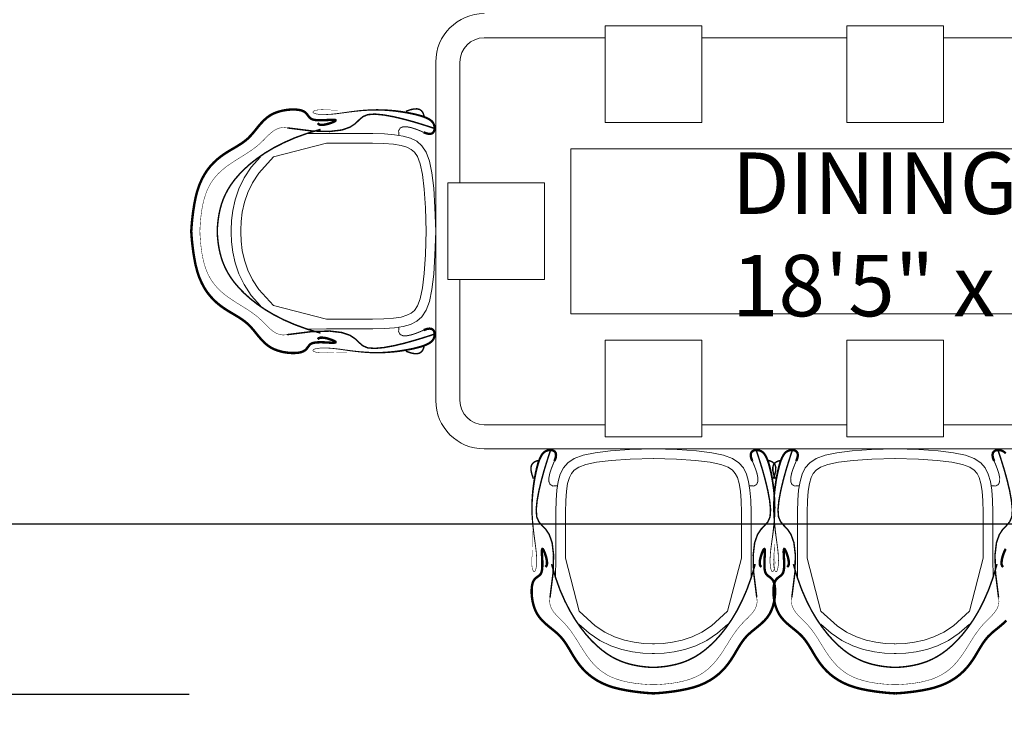
# Model space of a CAD drawing. Units: inches. Extents: x 870 to 1431, y 383 to 1070.
# Tile 4 of 9: x 1091 to 1171, y 661 to 718. Entities that reach past the tile are written whole.
import ezdxf

# ---------------------------------------------------------------- set-up
doc = ezdxf.new("R2010")
doc.units = ezdxf.units.IN
doc.header["$MEASUREMENT"] = 0
for name, color, linetype, lineweight in [('A-ANNO-DIMS', 2, 'Continuous', 18), ('A-AREA-IDEN', 7, 'Continuous', 25), ('A-FURN', 8, 'Continuous', 18)]:
    doc.layers.add(name, color=color, linetype=linetype, lineweight=lineweight)
doc.styles.get("Standard").update_dxf_attribs({"font": 'arial.ttf'})
doc.dimstyles.get("Standard").update_dxf_attribs({"dimtxt": 4, "dimasz": 0.18, "dimexe": 0.18, "dimexo": 0.0625, "dimgap": 0.09, "dimtad": 0, "dimtih": 1, "dimtoh": 1, "dimdec": 0, "dimrnd": 6, "dimzin": 0, "dimdsep": 46, "dimlunit": 3, "dimtxsty": 'Standard', "dimcen": 0.09, "dimadec": 0, "dimazin": 0, "dimtfac": 1, "dimtdec": 0, "dimtofl": 0, "dimtmove": 0, "dimatfit": 3, "dimfxl": 1, "dimtolj": 1, "dimtzin": 0, "dimarcsym": 0})

# ---------------------------------------------------------------- blocks, each defined once
blk = doc.blocks.new('ОГ53_на8персон_стол1900х900')
for p, q in [((-600, 54.3), (-600, 254.3)), ((-600, 254.3), (-400, 254.3)), ((-400, 254.3), (-400, 54.3)), ((-100, 254.3), (-100, 54.3)), ((100, 254.3), (-100, 254.3)), ((100, 54.3), (100, 254.3)), ((-850, 229.3), (-600, 229.3)), ((-400, 229.3), (-100, 229.3)), ((100, 229.3), (400, 229.3)), ((-950, -520.7), (-950, 179.3)), ((-900, -70.7), (-900, 179.3)), ((-400, 54.3), (-600, 54.3)), ((-100, 54.3), (100, 54.3)), ((670.7, 0), (-670.7, 0)), ((-670.7, 0), (-670.7, -341.4)), ((-725, -70.7), (-925, -70.7)), ((-925, -70.7), (-925, -270.7)), ((-725, -270.7), (-725, -70.7)), ((-925, -270.7), (-725, -270.7)), ((-900, -520.7), (-900, -270.7)), ((-670.7, -341.4), (670.7, -341.4)), ((-400, -395.7), (-600, -395.7)), ((-600, -395.7), (-600, -595.7)), ((-400, -595.7), (-400, -395.7)), ((-100, -595.7), (-100, -395.7)), ((-100, -395.7), (100, -395.7)), ((100, -395.7), (100, -595.7)), ((-600, -570.7), (-850, -570.7)), ((-100, -570.7), (-400, -570.7)), ((400, -570.7), (100, -570.7)), ((-600, -595.7), (-400, -595.7)), ((100, -595.7), (-100, -595.7)), ((850, -620.7), (-850, -620.7))]:
    blk.add_line(p, q)
for points, const_width in [([(-1194.1, 52.8), (-1192.1, 50.6), (-1188.9, 49.4), (-1184.9, 49.2), (-1180.3, 49.7), (-1175.5, 50.7), (-1170.8, 52), (-1166.4, 53.5), (-1162.7, 55), (-1159.9, 56.3), (-1158, 57.4), (-1157.1, 58.2), (-1157.1, 58.9), (-1158, 59.4), (-1159.8, 59.7), (-1162.5, 59.9), (-1166.1, 59.8), (-1170.5, 59.6), (-1175.5, 59.3), (-1181, 59), (-1186.6, 58.9), (-1192.2, 58.9), (-1197.5, 59.2), (-1202.2, 59.9), (-1206.2, 61.1), (-1209.2, 62.9), (-1211.5, 65), (-1213.4, 67.5), (-1215.3, 70.1), (-1217.4, 72.7), (-1219.9, 75.2), (-1223.4, 77.4), (-1227.9, 79.2), (-1233.8, 80.4), (-1240.9, 81.1), (-1248.8, 81.1), (-1257.3, 80.4), (-1266.1, 78.9), (-1274.9, 76.7), (-1283.4, 73.6), (-1291.3, 69.7), (-1298.4, 64.9), (-1304.8, 59.3), (-1310.7, 53.2), (-1316.3, 46.8), (-1321.6, 40.2), (-1326.9, 33.7), (-1332.4, 27.4), (-1338.1, 21.5), (-1344.4, 16.2), (-1351, 11.4), (-1358, 6.9), (-1365.2, 2.5), (-1372.6, -1.8), (-1380.1, -6.3), (-1387.6, -11.1), (-1395, -16.4), (-1402.3, -22.3), (-1409.4, -29), (-1416.2, -36.3), (-1422.7, -44.6), (-1428.7, -53.8), (-1434.1, -64), (-1439, -75.2), (-1443.2, -87.7), (-1446.7, -101.2), (-1449.4, -115.3), (-1451.6, -129.2), (-1453.2, -142.1), (-1454.4, -153.5), (-1455.1, -162.5), (-1455.5, -168.5), (-1455.7, -170.7)], 5), ([(-1011.7, 77.3), (-1002.5, 80.6), (-994.8, 82.3), (-988.5, 82.4), (-983.5, 81.2), (-979.7, 78.7), (-976.9, 75.1), (-975, 70.5), (-973.8, 65)], 3), ([(-1257.2, 43.1), (-1206.2, 36.7), (-1169.4, 35.7), (-1144.1, 38.7), (-1127.3, 44.6), (-1116.4, 51.9), (-1108.5, 59.6), (-1100.8, 66.2), (-1090.7, 70.5), (-1076, 71.6), (-1057.4, 69.8), (-1036.6, 66), (-1015.2, 60.9), (-994.5, 55.2), (-976.1, 49.6), (-961.6, 44.9), (-952.6, 41.8)], 3), ([(-1257.2, 43.1), (-1265.9, 43.9), (-1273.6, 42.7), (-1280.7, 39.8), (-1287.3, 35.6), (-1293.5, 30.4), (-1299.4, 24.7), (-1305.3, 18.6), (-1311.3, 12.7), (-1317.5, 7.2), (-1323.9, 2.1), (-1330.6, -2.8), (-1337.4, -7.4), (-1344.3, -11.8), (-1351.4, -16.3), (-1358.5, -20.7), (-1365.7, -25.2), (-1372.9, -29.9), (-1380, -34.9), (-1387, -40.2), (-1393.8, -45.9), (-1400.3, -52.2), (-1406.4, -59), (-1412.1, -66.5), (-1417.3, -74.8), (-1421.9, -83.9), (-1425.9, -94), (-1429.3, -105.1), (-1432.2, -117.4), (-1434.5, -130.9), (-1436.2, -145.8), (-1437.4, -162.1), (-1437.8, -170.7)], 1), ([(-1188.3, 40), (-1216.1, 31.7), (-1241.4, 22.5), (-1264.2, 12.5), (-1284.8, 2), (-1303.1, -8.9), (-1319.4, -20.1), (-1333.7, -31.3), (-1346.1, -42.5), (-1356.8, -53.5), (-1366, -64.2), (-1373.7, -74.7), (-1380.1, -84.9), (-1385.3, -94.9), (-1389.6, -104.7), (-1393, -114.3), (-1395.6, -123.7), (-1397.7, -132.7), (-1399.2, -141.4), (-1400.3, -149.3), (-1401, -156.4), (-1401.5, -162.3), (-1401.7, -166.8), (-1401.8, -169.6), (-1401.8, -170.7)], 3), ([(-974.9, 33.8), (-982.7, 37.2), (-991.6, 40.7), (-1001, 43.6), (-1010, 45.4), (-1017.8, 45.4), (-1023.6, 42.8), (-1026.8, 37.1), (-1026.4, 27.6)], 2), ([(-1194.1, -394.1), (-1192.1, -391.9), (-1188.9, -390.8), (-1184.9, -390.6), (-1180.3, -391.1), (-1175.5, -392), (-1170.8, -393.4), (-1166.4, -394.9), (-1162.7, -396.3), (-1159.9, -397.6), (-1158, -398.7), (-1157.1, -399.6), (-1157.1, -400.3), (-1158, -400.8), (-1159.8, -401.1), (-1162.5, -401.2), (-1166.1, -401.2), (-1170.5, -401), (-1175.5, -400.7), (-1181, -400.4), (-1186.6, -400.2), (-1192.2, -400.3), (-1197.5, -400.6), (-1202.2, -401.3), (-1206.2, -402.5), (-1209.2, -404.2), (-1211.5, -406.4), (-1213.4, -408.8), (-1215.3, -411.4), (-1217.4, -414.1), (-1219.9, -416.5), (-1223.4, -418.7), (-1227.9, -420.5), (-1233.8, -421.8), (-1240.9, -422.4), (-1248.8, -422.4), (-1257.3, -421.7), (-1266.1, -420.3), (-1274.9, -418), (-1283.4, -415), (-1291.3, -411), (-1298.4, -406.2), (-1304.8, -400.7), (-1310.7, -394.6), (-1316.3, -388.1), (-1321.6, -381.6), (-1326.9, -375), (-1332.4, -368.7), (-1338.1, -362.9), (-1344.4, -357.6), (-1351, -352.8), (-1358, -348.2), (-1365.2, -343.9), (-1372.6, -339.5), (-1380.1, -335), (-1387.6, -330.2), (-1395, -324.9), (-1402.3, -319), (-1409.4, -312.4), (-1416.2, -305), (-1422.7, -296.8), (-1428.7, -287.6), (-1434.1, -277.4), (-1439, -266.1), (-1443.2, -253.7), (-1446.7, -240.1), (-1449.4, -226.1), (-1451.6, -212.2), (-1453.2, -199.2), (-1454.4, -187.9), (-1455.1, -178.9), (-1455.5, -172.9), (-1455.7, -170.7)], 5), ([(-1257.2, -384.5), (-1265.9, -385.3), (-1273.6, -384), (-1280.7, -381.1), (-1287.3, -376.9), (-1293.5, -371.8), (-1299.4, -366), (-1305.3, -360), (-1311.3, -354.1), (-1317.5, -348.6), (-1323.9, -343.4), (-1330.6, -338.6), (-1337.4, -334), (-1344.3, -329.5), (-1351.4, -325.1), (-1358.5, -320.7), (-1365.7, -316.1), (-1372.9, -311.4), (-1380, -306.5), (-1387, -301.2), (-1393.8, -295.4), (-1400.3, -289.2), (-1406.4, -282.3), (-1412.1, -274.8), (-1417.3, -266.5), (-1421.9, -257.4), (-1425.9, -247.3), (-1429.3, -236.2), (-1432.2, -224), (-1434.5, -210.5), (-1436.2, -195.6), (-1437.4, -179.3), (-1437.8, -170.7)], 1), ([(-1188.3, -381.3), (-1216.1, -373), (-1241.4, -363.8), (-1264.2, -353.9), (-1284.8, -343.4), (-1303.1, -332.5), (-1319.4, -321.3), (-1333.7, -310), (-1346.1, -298.9), (-1356.8, -287.9), (-1366, -277.2), (-1373.7, -266.7), (-1380.1, -256.4), (-1385.3, -246.4), (-1389.6, -236.6), (-1393, -227), (-1395.6, -217.7), (-1397.7, -208.6), (-1399.2, -200), (-1400.3, -192), (-1401, -185), (-1401.5, -179.1), (-1401.7, -174.6), (-1401.8, -171.7), (-1401.8, -170.7)], 3), ([(-1257.2, -384.5), (-1206.2, -378.1), (-1169.4, -377.1), (-1144.1, -380.1), (-1127.3, -385.9), (-1116.4, -393.3), (-1108.5, -400.9), (-1100.8, -407.5), (-1090.7, -411.8), (-1076, -412.9), (-1057.4, -411.2), (-1036.6, -407.4), (-1015.2, -402.3), (-994.5, -396.5), (-976.1, -391), (-961.6, -386.3), (-952.6, -383.2)], 3), ([(-974.9, -375.1), (-982.7, -378.5), (-991.6, -382), (-1001, -385), (-1010, -386.8), (-1017.8, -386.7), (-1023.6, -384.2), (-1026.8, -378.4), (-1026.4, -368.9)], 2), ([(-1011.7, -418.7), (-1002.5, -422), (-994.8, -423.7), (-988.5, -423.8), (-983.5, -422.6), (-979.7, -420.1), (-976.9, -416.5), (-975, -411.9), (-973.8, -406.4)], 3), ([(-713.8, -927.9), (-707.4, -876.9), (-706.4, -840.1), (-709.4, -814.7), (-715.3, -798), (-722.6, -787), (-730.2, -779.2), (-736.8, -771.5), (-741.2, -761.4), (-742.3, -746.6), (-740.5, -728.1), (-736.7, -707.3), (-731.6, -685.8), (-725.9, -665.1), (-720.3, -646.8), (-715.6, -632.3), (-712.5, -623.2)], 3), ([(-286.2, -927.9), (-292.6, -876.9), (-293.6, -840.1), (-290.6, -814.7), (-284.7, -798), (-277.4, -787), (-269.8, -779.2), (-263.2, -771.5), (-258.8, -761.4), (-257.7, -746.6), (-259.5, -728.1), (-263.3, -707.3), (-268.4, -685.8), (-274.1, -665.1), (-279.7, -646.8), (-284.4, -632.3), (-287.5, -623.2)], 3), ([(-213.8, -927.9), (-207.4, -876.9), (-206.4, -840.1), (-209.4, -814.7), (-215.3, -798), (-222.6, -787), (-230.2, -779.2), (-236.8, -771.5), (-241.2, -761.4), (-242.3, -746.6), (-240.5, -728.1), (-236.7, -707.3), (-231.6, -685.8), (-225.9, -665.1), (-220.3, -646.8), (-215.6, -632.3), (-212.5, -623.2)], 3), ([(213.8, -927.9), (207.4, -876.9), (206.4, -840.1), (209.4, -814.7), (215.3, -798), (222.6, -787), (230.2, -779.2), (236.8, -771.5), (241.2, -761.4), (242.3, -746.6), (240.5, -728.1), (236.7, -707.3), (231.6, -685.8), (225.9, -665.1), (220.3, -646.8), (215.6, -632.3), (212.5, -623.2)], 3), ([(-748, -682.4), (-751.3, -673.2), (-753, -665.5), (-753.1, -659.2), (-751.9, -654.2), (-749.4, -650.4), (-745.8, -647.6), (-741.2, -645.6), (-735.7, -644.5)], 3), ([(-704.5, -645.6), (-707.8, -653.4), (-711.3, -662.3), (-714.3, -671.7), (-716.1, -680.7), (-716, -688.5), (-713.5, -694.3), (-707.8, -697.5), (-698.2, -697.1)], 2), ([(-295.5, -645.6), (-292.2, -653.4), (-288.7, -662.3), (-285.7, -671.7), (-283.9, -680.7), (-284, -688.5), (-286.5, -694.3), (-292.2, -697.5), (-301.8, -697.1)], 2), ([(-252, -682.4), (-248.7, -673.2), (-247, -665.5), (-246.9, -659.2), (-248.1, -654.2), (-250.6, -650.4), (-254.2, -647.6), (-258.8, -645.6), (-264.3, -644.5)], 3), ([(-248, -682.4), (-251.3, -673.2), (-253, -665.5), (-253.1, -659.2), (-251.9, -654.2), (-249.4, -650.4), (-245.8, -647.6), (-241.2, -645.6), (-235.7, -644.5)], 3), ([(-204.5, -645.6), (-207.8, -653.4), (-211.3, -662.3), (-214.3, -671.7), (-216.1, -680.7), (-216, -688.5), (-213.5, -694.3), (-207.8, -697.5), (-198.2, -697.1)], 2), ([(204.5, -645.6), (207.8, -653.4), (211.3, -662.3), (214.3, -671.7), (216.1, -680.7), (216, -688.5), (213.5, -694.3), (207.8, -697.5), (198.2, -697.1)], 2), ([(-723.4, -864.8), (-721.2, -862.7), (-720.1, -859.6), (-719.9, -855.5), (-720.4, -851), (-721.4, -846.2), (-722.7, -841.5), (-724.2, -837.1), (-725.7, -833.4), (-727, -830.6), (-728, -828.7), (-728.9, -827.8), (-729.6, -827.7), (-730.1, -828.6), (-730.4, -830.5), (-730.6, -833.2), (-730.5, -836.7), (-730.3, -841.2), (-730, -846.2), (-729.7, -851.7), (-729.6, -857.3), (-729.6, -862.9), (-729.9, -868.2), (-730.6, -872.9), (-731.8, -876.8), (-733.5, -879.9), (-735.7, -882.2), (-738.2, -884.1), (-740.8, -886), (-743.4, -888), (-745.9, -890.6), (-748.1, -894), (-749.8, -898.6), (-751.1, -904.5), (-751.7, -911.6), (-751.7, -919.5), (-751, -928), (-749.6, -936.8), (-747.4, -945.6), (-744.3, -954.1), (-740.4, -962), (-735.5, -969.1), (-730, -975.5), (-723.9, -981.4), (-717.5, -986.9), (-710.9, -992.3), (-704.3, -997.6), (-698.1, -1003), (-692.2, -1008.8), (-686.9, -1015.1), (-682.1, -1021.7), (-677.6, -1028.7), (-673.2, -1035.9), (-668.9, -1043.3), (-664.4, -1050.8), (-659.5, -1058.3), (-654.2, -1065.7), (-648.3, -1073), (-641.7, -1080.1), (-634.3, -1086.9), (-626.1, -1093.3), (-616.9, -1099.3), (-606.7, -1104.8), (-595.4, -1109.7), (-583, -1113.9), (-569.5, -1117.3), (-555.4, -1120.1), (-541.5, -1122.3), (-528.6, -1123.9), (-517.2, -1125.1), (-508.2, -1125.8), (-502.2, -1126.2), (-500, -1126.3)], 5), ([(-276.6, -864.8), (-278.8, -862.7), (-279.9, -859.6), (-280.1, -855.5), (-279.6, -851), (-278.6, -846.2), (-277.3, -841.5), (-275.8, -837.1), (-274.3, -833.4), (-273, -830.6), (-272, -828.7), (-271.1, -827.8), (-270.4, -827.7), (-269.9, -828.6), (-269.6, -830.5), (-269.4, -833.2), (-269.5, -836.7), (-269.7, -841.2), (-270, -846.2), (-270.3, -851.7), (-270.4, -857.3), (-270.4, -862.9), (-270.1, -868.2), (-269.4, -872.9), (-268.2, -876.8), (-266.5, -879.9), (-264.3, -882.2), (-261.8, -884.1), (-259.2, -886), (-256.6, -888), (-254.1, -890.6), (-251.9, -894), (-250.2, -898.6), (-248.9, -904.5), (-248.3, -911.6), (-248.3, -919.5), (-249, -928), (-250.4, -936.8), (-252.6, -945.6), (-255.7, -954.1), (-259.6, -962), (-264.5, -969.1), (-270, -975.5), (-276.1, -981.4), (-282.5, -986.9), (-289.1, -992.3), (-295.7, -997.6), (-301.9, -1003), (-307.8, -1008.8), (-313.1, -1015.1), (-317.9, -1021.7), (-322.4, -1028.7), (-326.8, -1035.9), (-331.1, -1043.3), (-335.6, -1050.8), (-340.5, -1058.3), (-345.8, -1065.7), (-351.7, -1073), (-358.3, -1080.1), (-365.7, -1086.9), (-373.9, -1093.3), (-383.1, -1099.3), (-393.3, -1104.8), (-404.6, -1109.7), (-417, -1113.9), (-430.5, -1117.3), (-444.6, -1120.1), (-458.5, -1122.3), (-471.4, -1123.9), (-482.8, -1125.1), (-491.8, -1125.8), (-497.8, -1126.2), (-500, -1126.3)], 5), ([(-223.4, -864.8), (-221.2, -862.7), (-220.1, -859.6), (-219.9, -855.5), (-220.4, -851), (-221.4, -846.2), (-222.7, -841.5), (-224.2, -837.1), (-225.7, -833.4), (-227, -830.6), (-228, -828.7), (-228.9, -827.8), (-229.6, -827.7), (-230.1, -828.6), (-230.4, -830.5), (-230.6, -833.2), (-230.5, -836.7), (-230.3, -841.2), (-230, -846.2), (-229.7, -851.7), (-229.6, -857.3), (-229.6, -862.9), (-229.9, -868.2), (-230.6, -872.9), (-231.8, -876.8), (-233.5, -879.9), (-235.7, -882.2), (-238.2, -884.1), (-240.8, -886), (-243.4, -888), (-245.9, -890.6), (-248.1, -894), (-249.8, -898.6), (-251.1, -904.5), (-251.7, -911.6), (-251.7, -919.5), (-251, -928), (-249.6, -936.8), (-247.4, -945.6), (-244.3, -954.1), (-240.4, -962), (-235.5, -969.1), (-230, -975.5), (-223.9, -981.4), (-217.5, -986.9), (-210.9, -992.3), (-204.3, -997.6), (-198.1, -1003), (-192.2, -1008.8), (-186.9, -1015.1), (-182.1, -1021.7), (-177.6, -1028.7), (-173.2, -1035.9), (-168.9, -1043.3), (-164.4, -1050.8), (-159.5, -1058.3), (-154.2, -1065.7), (-148.3, -1073), (-141.7, -1080.1), (-134.3, -1086.9), (-126.1, -1093.3), (-116.9, -1099.3), (-106.7, -1104.8), (-95.4, -1109.7), (-83, -1113.9), (-69.5, -1117.3), (-55.4, -1120.1), (-41.5, -1122.3), (-28.6, -1123.9), (-17.2, -1125.1), (-8.2, -1125.8), (-2.2, -1126.2), (0, -1126.3)], 5), ([(223.4, -864.8), (221.2, -862.7), (220.1, -859.6), (219.9, -855.5), (220.4, -851), (221.4, -846.2), (222.7, -841.5), (224.2, -837.1), (225.7, -833.4), (227, -830.6), (228, -828.7), (228.9, -827.8)], 5), ([(230, -975.5), (223.9, -981.4), (217.5, -986.9), (210.9, -992.3), (204.3, -997.6), (198.1, -1003), (192.2, -1008.8), (186.9, -1015.1), (182.1, -1021.7), (177.6, -1028.7), (173.2, -1035.9), (168.9, -1043.3), (164.4, -1050.8), (159.5, -1058.3), (154.2, -1065.7), (148.3, -1073), (141.7, -1080.1), (134.3, -1086.9), (126.1, -1093.3), (116.9, -1099.3), (106.7, -1104.8), (95.4, -1109.7), (83, -1113.9), (69.5, -1117.3), (55.4, -1120.1), (41.5, -1122.3), (28.6, -1123.9), (17.2, -1125.1), (8.2, -1125.8), (2.2, -1126.2), (0, -1126.3)], 5), ([(-710.6, -859), (-702.3, -886.8), (-693.2, -912.1), (-683.2, -934.9), (-672.7, -955.5), (-661.8, -973.8), (-650.6, -990), (-639.4, -1004.3), (-628.2, -1016.8), (-617.2, -1027.5), (-606.5, -1036.7), (-596, -1044.4), (-585.8, -1050.8), (-575.7, -1056), (-565.9, -1060.3), (-556.4, -1063.6), (-547, -1066.3), (-537.9, -1068.3), (-529.3, -1069.9), (-521.3, -1071), (-514.3, -1071.7), (-508.4, -1072.2), (-503.9, -1072.4), (-501, -1072.5), (-500, -1072.5)], 3), ([(-289.4, -859), (-297.7, -886.8), (-306.8, -912.1), (-316.8, -934.9), (-327.3, -955.5), (-338.2, -973.8), (-349.4, -990), (-360.6, -1004.3), (-371.8, -1016.8), (-382.8, -1027.5), (-393.5, -1036.7), (-404, -1044.4), (-414.2, -1050.8), (-424.3, -1056), (-434.1, -1060.3), (-443.6, -1063.6), (-453, -1066.3), (-462.1, -1068.3), (-470.7, -1069.9), (-478.7, -1071), (-485.7, -1071.7), (-491.6, -1072.2), (-496.1, -1072.4), (-499, -1072.5), (-500, -1072.5)], 3), ([(-210.6, -859), (-202.3, -886.8), (-193.2, -912.1), (-183.2, -934.9), (-172.7, -955.5), (-161.8, -973.8), (-150.6, -990), (-139.4, -1004.3), (-128.2, -1016.8), (-117.2, -1027.5), (-106.5, -1036.7), (-96, -1044.4), (-85.8, -1050.8), (-75.7, -1056), (-65.9, -1060.3), (-56.4, -1063.6), (-47, -1066.3), (-37.9, -1068.3), (-29.3, -1069.9), (-21.3, -1071), (-14.3, -1071.7), (-8.4, -1072.2), (-3.9, -1072.4), (-1, -1072.5), (0, -1072.5)], 3), ([(210.6, -859), (202.3, -886.8), (193.2, -912.1), (183.2, -934.9), (172.7, -955.5), (161.8, -973.8), (150.6, -990), (139.4, -1004.3), (128.2, -1016.8), (117.2, -1027.5), (106.5, -1036.7), (96, -1044.4), (85.8, -1050.8), (75.7, -1056), (65.9, -1060.3), (56.4, -1063.6), (47, -1066.3), (37.9, -1068.3), (29.3, -1069.9), (21.3, -1071), (14.3, -1071.7), (8.4, -1072.2), (3.9, -1072.4), (1, -1072.5), (0, -1072.5)], 3), ([(-713.8, -927.9), (-714.6, -936.5), (-713.4, -944.3), (-710.5, -951.4), (-706.3, -958), (-701.1, -964.1), (-695.3, -970.1), (-689.3, -976), (-683.4, -982), (-677.9, -988.2), (-672.8, -994.6), (-667.9, -1001.3), (-663.3, -1008.1), (-658.8, -1015), (-654.4, -1022.1), (-650, -1029.2), (-645.5, -1036.4), (-640.8, -1043.6), (-635.8, -1050.7), (-630.5, -1057.7), (-624.7, -1064.5), (-618.5, -1071), (-611.7, -1077.1), (-604.1, -1082.8), (-595.9, -1088), (-586.7, -1092.6), (-576.7, -1096.6), (-565.5, -1100), (-553.3, -1102.9), (-539.8, -1105.2), (-524.9, -1106.9), (-508.6, -1108.1), (-500, -1108.4)], 1), ([(-286.2, -927.9), (-285.4, -936.5), (-286.6, -944.3), (-289.5, -951.4), (-293.7, -958), (-298.9, -964.1), (-304.7, -970.1), (-310.7, -976), (-316.6, -982), (-322.1, -988.2), (-327.2, -994.6), (-332.1, -1001.3), (-336.7, -1008.1), (-341.2, -1015), (-345.6, -1022.1), (-350, -1029.2), (-354.5, -1036.4), (-359.2, -1043.6), (-364.2, -1050.7), (-369.5, -1057.7), (-375.3, -1064.5), (-381.5, -1071), (-388.3, -1077.1), (-395.9, -1082.8), (-404.1, -1088), (-413.3, -1092.6), (-423.3, -1096.6), (-434.5, -1100), (-446.7, -1102.9), (-460.2, -1105.2), (-475.1, -1106.9), (-491.4, -1108.1), (-500, -1108.4)], 1), ([(-213.8, -927.9), (-214.6, -936.5), (-213.4, -944.3), (-210.5, -951.4), (-206.3, -958), (-201.1, -964.1), (-195.3, -970.1), (-189.3, -976), (-183.4, -982), (-177.9, -988.2), (-172.8, -994.6), (-167.9, -1001.3), (-163.3, -1008.1), (-158.8, -1015), (-154.4, -1022.1), (-150, -1029.2), (-145.5, -1036.4), (-140.8, -1043.6), (-135.8, -1050.7), (-130.5, -1057.7), (-124.7, -1064.5), (-118.5, -1071), (-111.7, -1077.1), (-104.1, -1082.8), (-95.9, -1088), (-86.7, -1092.6), (-76.7, -1096.6), (-65.5, -1100), (-53.3, -1102.9), (-39.8, -1105.2), (-24.9, -1106.9), (-8.6, -1108.1), (0, -1108.4)], 1), ([(213.8, -927.9), (214.6, -936.5), (213.4, -944.3), (210.5, -951.4), (206.3, -958), (201.1, -964.1), (195.3, -970.1), (189.3, -976), (183.4, -982), (177.9, -988.2), (172.8, -994.6), (167.9, -1001.3), (163.3, -1008.1), (158.8, -1015), (154.4, -1022.1), (150, -1029.2), (145.5, -1036.4), (140.8, -1043.6), (135.8, -1050.7), (130.5, -1057.7), (124.7, -1064.5), (118.5, -1071), (111.7, -1077.1), (104.1, -1082.8), (95.9, -1088), (86.7, -1092.6), (76.7, -1096.6), (65.5, -1100), (53.3, -1102.9), (39.8, -1105.2), (24.9, -1106.9), (8.6, -1108.1), (0, -1108.4)], 1)]:
    blk.add_lwpolyline(points, dxfattribs=dict(const_width=const_width))
for points in [[(-974.9, 33.8, 5, 4.91, 0), (-968.1, 31.4, 4.91, 4.84, 0), (-962.8, 30.6, 4.84, 4.78, 0), (-958.7, 31.2, 4.78, 4.74, 0), (-955.8, 33, 4.74, 4.7, 0), (-953.9, 35.6, 4.7, 4.65, 0), (-952.9, 38.8, 4.65, 4.61, 0), (-952.5, 42.3, 4.61, 4.56, 0), (-952.8, 45.8, 4.56, 4.52, 0), (-953.5, 49.1, 4.52, 4.47, 0), (-954.8, 52.2, 4.47, 4.43, 0), (-956.7, 55.2, 4.43, 4.38, 0), (-959.5, 58, 4.38, 4.32, 0), (-963.2, 60.6, 4.32, 4.25, 0), (-967.9, 63.2, 4.25, 4.17, 0), (-973.8, 65.6, 4.17, 4.07, 0), (-981, 68, 4.07, 3.95, 0), (-989.6, 70.4, 3.95, 3.82, 0), (-999.3, 72.6, 3.82, 3.68, 0), (-1010.1, 74.7, 3.68, 3.53, 0), (-1021.6, 76.5, 3.53, 3.37, 0), (-1033.7, 78.1, 3.37, 3.21, 0), (-1046.2, 79.3, 3.21, 3.05, 0), (-1058.8, 80.1, 3.05, 2.88, 0), (-1071.4, 80.4, 2.88, 2.72, 0), (-1083.8, 80.2, 2.72, 2.57, 0), (-1095.8, 79.5, 2.57, 2.41, 0), (-1107.4, 78.6, 2.41, 2.27, 0), (-1118.5, 77.3, 2.27, 2.13, 0), (-1129, 76, 2.13, 2, 0), (-1138.9, 74.6, 2, 1.88, 0), (-1148, 73.4, 1.88, 1.78, 0), (-1156.3, 72.3, 1.78, 1.68, 0), (-1163.7, 71.5, 1.68, 1.59, 0), (-1170.3, 71, 1.59, 1.52, 0), (-1176.1, 70.7, 1.52, 1.45, 0), (-1181.2, 70.7, 1.45, 1.4, 0), (-1185.6, 70.7, 1.4, 1.35, 0), (-1189.4, 71, 1.35, 1.3, 0), (-1192.6, 71.3, 1.3, 1.27, 0), (-1195.3, 71.7, 1.27, 1.24, 0), (-1197.6, 72.1, 1.24, 1.21, 0), (-1199.5, 72.6, 1.21, 1.19, 0), (-1201, 73.1, 1.19, 1.18, 0), (-1202.2, 73.6, 1.18, 1.16, 0), (-1203, 74.1, 1.16, 1.15, 0), (-1203.6, 74.6, 1.15, 1.14, 0), (-1203.9, 75.1, 1.14, 1.14, 0), (-1204, 75.6, 1.14, 1.13, 0), (-1203.9, 76.2, 1.13, 1.12, 0), (-1203.6, 76.6, 1.12, 1.12, 0), (-1203.2, 77.1, 1.12, 1.11, 0), (-1202.6, 77.6, 1.11, 1.09, 0), (-1201.8, 78, 1.09, 1.08, 0), (-1200.9, 78.4, 1.08, 1.07, 0), (-1199.8, 78.9, 1.07, 1.05, 0), (-1198.6, 79.2, 1.05, 1.03, 0), (-1197.2, 79.6, 1.03, 1.01, 0), (-1195.6, 79.9, 1.01, 0.986, 0), (-1193.8, 80.2, 0.986, 0.959, 0), (-1191.7, 80.4, 0.959, 0.926, 0), (-1189.2, 80.6, 0.926, 0.889, 0), (-1186.3, 80.7, 0.889, 0.846, 0), (-1183, 80.7, 0.846, 0.796, 0), (-1179.1, 80.6, 0.796, 0.738, 0), (-1174.7, 80.4, 0.738, 0.672, 0), (-1169.6, 80.2, 0.672, 0.595, 0), (-1163.7, 79.9, 0.595, 0.506, 0), (-1156.8, 79.6, 0.506, 0.404, 0), (-1148.9, 79.4, 0.404, 0.286, 0), (-1139.9, 79.2, 0.286, 0.152, 0), (-1129.5, 79.2, 0.152, 0, 0), (-1117.8, 79.4, 0, 0, 0)], [(-974.9, -375.1, 5, 4.91, 0), (-968.1, -372.7, 4.91, 4.84, 0), (-962.8, -372, 4.84, 4.78, 0), (-958.7, -372.6, 4.78, 4.74, 0), (-955.8, -374.3, 4.74, 4.7, 0), (-953.9, -376.9, 4.7, 4.65, 0), (-952.9, -380.1, 4.65, 4.61, 0), (-952.5, -383.6, 4.61, 4.56, 0), (-952.8, -387.1, 4.56, 4.52, 0), (-953.5, -390.5, 4.52, 4.47, 0), (-954.8, -393.6, 4.47, 4.43, 0), (-956.7, -396.6, 4.43, 4.38, 0), (-959.5, -399.3, 4.38, 4.32, 0), (-963.2, -402, 4.32, 4.25, 0), (-967.9, -404.5, 4.25, 4.17, 0), (-973.8, -407, 4.17, 4.07, 0), (-981, -409.4, 4.07, 3.95, 0), (-989.6, -411.7, 3.95, 3.82, 0), (-999.3, -414, 3.82, 3.68, 0), (-1010.1, -416, 3.68, 3.53, 0), (-1021.6, -417.9, 3.53, 3.37, 0), (-1033.7, -419.5, 3.37, 3.21, 0), (-1046.2, -420.7, 3.21, 3.05, 0), (-1058.8, -421.5, 3.05, 2.88, 0), (-1071.4, -421.8, 2.88, 2.72, 0), (-1083.8, -421.6, 2.72, 2.57, 0), (-1095.8, -420.9, 2.57, 2.41, 0), (-1107.4, -419.9, 2.41, 2.27, 0), (-1118.5, -418.7, 2.27, 2.13, 0), (-1129, -417.4, 2.13, 2, 0), (-1138.9, -416, 2, 1.88, 0), (-1148, -414.7, 1.88, 1.78, 0), (-1156.3, -413.7, 1.78, 1.68, 0), (-1163.7, -412.9, 1.68, 1.59, 0), (-1170.3, -412.4, 1.59, 1.52, 0), (-1176.1, -412.1, 1.52, 1.45, 0), (-1181.2, -412, 1.45, 1.4, 0), (-1185.6, -412.1, 1.4, 1.35, 0), (-1189.4, -412.3, 1.35, 1.3, 0), (-1192.6, -412.7, 1.3, 1.27, 0), (-1195.3, -413, 1.27, 1.24, 0), (-1197.6, -413.5, 1.24, 1.21, 0), (-1199.5, -413.9, 1.21, 1.19, 0), (-1201, -414.4, 1.19, 1.18, 0), (-1202.2, -414.9, 1.18, 1.16, 0), (-1203, -415.4, 1.16, 1.15, 0), (-1203.6, -416, 1.15, 1.14, 0), (-1203.9, -416.5, 1.14, 1.14, 0), (-1204, -417, 1.14, 1.13, 0), (-1203.9, -417.5, 1.13, 1.12, 0), (-1203.6, -418, 1.12, 1.12, 0), (-1203.2, -418.5, 1.12, 1.11, 0), (-1202.6, -418.9, 1.11, 1.09, 0), (-1201.8, -419.4, 1.09, 1.08, 0), (-1200.9, -419.8, 1.08, 1.07, 0), (-1199.8, -420.2, 1.07, 1.05, 0), (-1198.6, -420.6, 1.05, 1.03, 0), (-1197.2, -421, 1.03, 1.01, 0), (-1195.6, -421.3, 1.01, 0.986, 0), (-1193.8, -421.6, 0.986, 0.959, 0), (-1191.7, -421.8, 0.959, 0.926, 0), (-1189.2, -422, 0.926, 0.889, 0), (-1186.3, -422, 0.889, 0.846, 0), (-1183, -422, 0.846, 0.796, 0), (-1179.1, -422, 0.796, 0.738, 0), (-1174.7, -421.8, 0.738, 0.672, 0), (-1169.6, -421.5, 0.672, 0.595, 0), (-1163.7, -421.2, 0.595, 0.506, 0), (-1156.8, -421, 0.506, 0.404, 0), (-1148.9, -420.7, 0.404, 0.286, 0), (-1139.9, -420.6, 0.286, 0.152, 0), (-1129.5, -420.6, 0.152, 0, 0), (-1117.8, -420.7, 0, 0, 0)], [(-704.5, -645.6, 5, 4.91, 0), (-702, -638.8, 4.91, 4.84, 0), (-701.3, -633.5, 4.84, 4.78, 0), (-701.9, -629.4, 4.78, 4.74, 0), (-703.7, -626.5, 4.74, 4.7, 0), (-706.3, -624.6, 4.7, 4.65, 0), (-709.4, -623.5, 4.65, 4.61, 0), (-712.9, -623.2, 4.61, 4.56, 0), (-716.5, -623.5, 4.56, 4.52, 0), (-719.8, -624.2, 4.52, 4.47, 0), (-722.9, -625.5, 4.47, 4.43, 0), (-725.9, -627.4, 4.43, 4.38, 0), (-728.7, -630.2, 4.38, 4.32, 0), (-731.3, -633.9, 4.32, 4.25, 0), (-733.8, -638.6, 4.25, 4.17, 0), (-736.3, -644.5, 4.17, 4.07, 0), (-738.7, -651.7, 4.07, 3.95, 0), (-741, -660.3, 3.95, 3.82, 0), (-743.3, -670, 3.82, 3.68, 0), (-745.4, -680.8, 3.68, 3.53, 0), (-747.2, -692.3, 3.53, 3.37, 0), (-748.8, -704.4, 3.37, 3.21, 0), (-750, -716.9, 3.21, 3.05, 0), (-750.8, -729.5, 3.05, 2.88, 0), (-751.1, -742.1, 2.88, 2.72, 0), (-750.9, -754.5, 2.72, 2.57, 0), (-750.2, -766.5, 2.57, 2.41, 0), (-749.2, -778.1, 2.41, 2.27, 0), (-748, -789.2, 2.27, 2.13, 0), (-746.7, -799.7, 2.13, 2, 0), (-745.3, -809.6, 2, 1.88, 0), (-744.1, -818.7, 1.88, 1.78, 0), (-743, -827, 1.78, 1.68, 0), (-742.2, -834.4, 1.68, 1.59, 0), (-741.7, -841, 1.59, 1.52, 0), (-741.4, -846.8, 1.52, 1.45, 0), (-741.3, -851.9, 1.45, 1.4, 0), (-741.4, -856.3, 1.4, 1.35, 0), (-741.6, -860.1, 1.35, 1.3, 0), (-742, -863.3, 1.3, 1.27, 0), (-742.4, -866, 1.27, 1.24, 0), (-742.8, -868.3, 1.24, 1.21, 0), (-743.3, -870.2, 1.21, 1.19, 0), (-743.8, -871.7, 1.19, 1.18, 0), (-744.3, -872.9, 1.18, 1.16, 0), (-744.8, -873.7, 1.16, 1.15, 0), (-745.3, -874.3, 1.15, 1.14, 0), (-745.8, -874.6, 1.14, 1.14, 0), (-746.3, -874.7, 1.14, 1.13, 0), (-746.8, -874.6, 1.13, 1.12, 0), (-747.3, -874.3, 1.12, 1.12, 0), (-747.8, -873.9, 1.12, 1.11, 0), (-748.3, -873.3, 1.11, 1.09, 0), (-748.7, -872.5, 1.09, 1.08, 0), (-749.1, -871.6, 1.08, 1.07, 0), (-749.5, -870.5, 1.07, 1.05, 0), (-749.9, -869.2, 1.05, 1.03, 0), (-750.3, -867.9, 1.03, 1.01, 0), (-750.6, -866.3, 1.01, 0.986, 0), (-750.9, -864.5, 0.986, 0.959, 0), (-751.1, -862.4, 0.959, 0.926, 0), (-751.3, -859.9, 0.926, 0.889, 0), (-751.4, -857, 0.889, 0.846, 0), (-751.4, -853.7, 0.846, 0.796, 0), (-751.3, -849.8, 0.796, 0.738, 0), (-751.1, -845.4, 0.738, 0.672, 0), (-750.8, -840.3, 0.672, 0.595, 0), (-750.6, -834.3, 0.595, 0.506, 0), (-750.3, -827.5, 0.506, 0.404, 0), (-750.1, -819.6, 0.404, 0.286, 0), (-749.9, -810.5, 0.286, 0.152, 0), (-749.9, -800.2, 0.152, 0, 0), (-750, -788.5, 0, 0, 0)], [(-295.5, -645.6, 5, 4.91, 0), (-298, -638.8, 4.91, 4.84, 0), (-298.7, -633.5, 4.84, 4.78, 0), (-298.1, -629.4, 4.78, 4.74, 0), (-296.3, -626.5, 4.74, 4.7, 0), (-293.7, -624.6, 4.7, 4.65, 0), (-290.6, -623.5, 4.65, 4.61, 0), (-287.1, -623.2, 4.61, 4.56, 0), (-283.5, -623.5, 4.56, 4.52, 0), (-280.2, -624.2, 4.52, 4.47, 0), (-277.1, -625.5, 4.47, 4.43, 0), (-274.1, -627.4, 4.43, 4.38, 0), (-271.3, -630.2, 4.38, 4.32, 0), (-268.7, -633.9, 4.32, 4.25, 0), (-266.2, -638.6, 4.25, 4.17, 0), (-263.7, -644.5, 4.17, 4.07, 0), (-261.3, -651.7, 4.07, 3.95, 0), (-259, -660.3, 3.95, 3.82, 0), (-256.7, -670, 3.82, 3.68, 0), (-254.6, -680.8, 3.68, 3.53, 0), (-252.8, -692.3, 3.53, 3.37, 0), (-251.2, -704.4, 3.37, 3.21, 0), (-250, -716.9, 3.21, 3.05, 0), (-249.2, -729.5, 3.05, 2.88, 0), (-248.9, -742.1, 2.88, 2.72, 0), (-249.1, -754.5, 2.72, 2.57, 0), (-249.8, -766.5, 2.57, 2.41, 0), (-250.8, -778.1, 2.41, 2.27, 0), (-252, -789.2, 2.27, 2.13, 0), (-253.3, -799.7, 2.13, 2, 0), (-254.7, -809.6, 2, 1.88, 0), (-255.9, -818.7, 1.88, 1.78, 0), (-257, -827, 1.78, 1.68, 0), (-257.8, -834.4, 1.68, 1.59, 0), (-258.3, -841, 1.59, 1.52, 0), (-258.6, -846.8, 1.52, 1.45, 0), (-258.7, -851.9, 1.45, 1.4, 0), (-258.6, -856.3, 1.4, 1.35, 0), (-258.4, -860.1, 1.35, 1.3, 0), (-258, -863.3, 1.3, 1.27, 0), (-257.6, -866, 1.27, 1.24, 0), (-257.2, -868.3, 1.24, 1.21, 0), (-256.7, -870.2, 1.21, 1.19, 0), (-256.2, -871.7, 1.19, 1.18, 0), (-255.7, -872.9, 1.18, 1.16, 0), (-255.2, -873.7, 1.16, 1.15, 0), (-254.7, -874.3, 1.15, 1.14, 0), (-254.2, -874.6, 1.14, 1.14, 0), (-253.7, -874.7, 1.14, 1.13, 0), (-253.2, -874.6, 1.13, 1.12, 0), (-252.7, -874.3, 1.12, 1.12, 0), (-252.2, -873.9, 1.12, 1.11, 0), (-251.7, -873.3, 1.11, 1.09, 0), (-251.3, -872.5, 1.09, 1.08, 0), (-250.9, -871.6, 1.08, 1.07, 0), (-250.5, -870.5, 1.07, 1.05, 0), (-250.1, -869.2, 1.05, 1.03, 0), (-249.7, -867.9, 1.03, 1.01, 0), (-249.4, -866.3, 1.01, 0.986, 0), (-249.1, -864.5, 0.986, 0.959, 0), (-248.9, -862.4, 0.959, 0.926, 0), (-248.7, -859.9, 0.926, 0.889, 0), (-248.6, -857, 0.889, 0.846, 0), (-248.6, -853.7, 0.846, 0.796, 0), (-248.7, -849.8, 0.796, 0.738, 0), (-248.9, -845.4, 0.738, 0.672, 0), (-249.2, -840.3, 0.672, 0.595, 0), (-249.4, -834.3, 0.595, 0.506, 0), (-249.7, -827.5, 0.506, 0.404, 0), (-249.9, -819.6, 0.404, 0.286, 0), (-250.1, -810.5, 0.286, 0.152, 0), (-250.1, -800.2, 0.152, 0, 0), (-250, -788.5, 0, 0, 0)], [(-204.5, -645.6, 5, 4.91, 0), (-202, -638.8, 4.91, 4.84, 0), (-201.3, -633.5, 4.84, 4.78, 0), (-201.9, -629.4, 4.78, 4.74, 0), (-203.7, -626.5, 4.74, 4.7, 0), (-206.3, -624.6, 4.7, 4.65, 0), (-209.4, -623.5, 4.65, 4.61, 0), (-212.9, -623.2, 4.61, 4.56, 0), (-216.5, -623.5, 4.56, 4.52, 0), (-219.8, -624.2, 4.52, 4.47, 0), (-222.9, -625.5, 4.47, 4.43, 0), (-225.9, -627.4, 4.43, 4.38, 0), (-228.7, -630.2, 4.38, 4.32, 0), (-231.3, -633.9, 4.32, 4.25, 0), (-233.8, -638.6, 4.25, 4.17, 0), (-236.3, -644.5, 4.17, 4.07, 0), (-238.7, -651.7, 4.07, 3.95, 0), (-241, -660.3, 3.95, 3.82, 0), (-243.3, -670, 3.82, 3.68, 0), (-245.4, -680.8, 3.68, 3.53, 0), (-247.2, -692.3, 3.53, 3.37, 0), (-248.8, -704.4, 3.37, 3.21, 0), (-250, -716.9, 3.21, 3.05, 0), (-250.8, -729.5, 3.05, 2.88, 0), (-251.1, -742.1, 2.88, 2.72, 0), (-250.9, -754.5, 2.72, 2.57, 0), (-250.2, -766.5, 2.57, 2.41, 0), (-249.2, -778.1, 2.41, 2.27, 0), (-248, -789.2, 2.27, 2.13, 0), (-246.7, -799.7, 2.13, 2, 0), (-245.3, -809.6, 2, 1.88, 0), (-244.1, -818.7, 1.88, 1.78, 0), (-243, -827, 1.78, 1.68, 0), (-242.2, -834.4, 1.68, 1.59, 0), (-241.7, -841, 1.59, 1.52, 0), (-241.4, -846.8, 1.52, 1.45, 0), (-241.3, -851.9, 1.45, 1.4, 0), (-241.4, -856.3, 1.4, 1.35, 0), (-241.6, -860.1, 1.35, 1.3, 0), (-242, -863.3, 1.3, 1.27, 0), (-242.4, -866, 1.27, 1.24, 0), (-242.8, -868.3, 1.24, 1.21, 0), (-243.3, -870.2, 1.21, 1.19, 0), (-243.8, -871.7, 1.19, 1.18, 0), (-244.3, -872.9, 1.18, 1.16, 0), (-244.8, -873.7, 1.16, 1.15, 0), (-245.3, -874.3, 1.15, 1.14, 0), (-245.8, -874.6, 1.14, 1.14, 0), (-246.3, -874.7, 1.14, 1.13, 0), (-246.8, -874.6, 1.13, 1.12, 0), (-247.3, -874.3, 1.12, 1.12, 0), (-247.8, -873.9, 1.12, 1.11, 0), (-248.3, -873.3, 1.11, 1.09, 0), (-248.7, -872.5, 1.09, 1.08, 0), (-249.1, -871.6, 1.08, 1.07, 0), (-249.5, -870.5, 1.07, 1.05, 0), (-249.9, -869.2, 1.05, 1.03, 0), (-250.3, -867.9, 1.03, 1.01, 0), (-250.6, -866.3, 1.01, 0.986, 0), (-250.9, -864.5, 0.986, 0.959, 0), (-251.1, -862.4, 0.959, 0.926, 0), (-251.3, -859.9, 0.926, 0.889, 0), (-251.4, -857, 0.889, 0.846, 0), (-251.4, -853.7, 0.846, 0.796, 0), (-251.3, -849.8, 0.796, 0.738, 0), (-251.1, -845.4, 0.738, 0.672, 0), (-250.8, -840.3, 0.672, 0.595, 0), (-250.6, -834.3, 0.595, 0.506, 0), (-250.3, -827.5, 0.506, 0.404, 0), (-250.1, -819.6, 0.404, 0.286, 0), (-249.9, -810.5, 0.286, 0.152, 0), (-249.9, -800.2, 0.152, 0, 0), (-250, -788.5, 0, 0, 0)], [(204.5, -645.6, 5, 4.91, 0), (202, -638.8, 4.91, 4.84, 0), (201.3, -633.5, 4.84, 4.78, 0), (201.9, -629.4, 4.78, 4.74, 0), (203.7, -626.5, 4.74, 4.7, 0), (206.3, -624.6, 4.7, 4.65, 0), (209.4, -623.5, 4.65, 4.61, 0), (212.9, -623.2, 4.61, 4.56, 0), (216.5, -623.5, 4.56, 4.52, 0), (219.8, -624.2, 4.52, 4.47, 0), (222.9, -625.5, 4.47, 4.43, 0), (225.9, -627.4, 4.43, 4.38, 0), (228.7, -630.2, 4.38, 4.32, 0)]]:
    blk.add_lwpolyline(points, format="xyseb")
for points in [[(-1216.1, 31.7), (-1175.8, 31.2), (-1139.9, 31.2), (-1108.2, 31.3), (-1080.4, 31.2), (-1056.3, 30.5), (-1035.4, 29), (-1017.4, 26.2), (-1002.2, 21.8), (-989.4, 15.4), (-978.7, 6.1), (-970.1, -7.2), (-963.2, -25.6), (-958, -50.1), (-954.2, -81.7), (-951.6, -121.6), (-950, -170.7)], [(-1285.7, -17.1), (-1175.9, 11.2), (-1139.9, 11.2), (-1108.2, 11.3), (-1080.8, 11.2), (-1057.3, 10.5), (-1037.6, 9.1), (-1021.7, 6.6), (-1009.5, 3.1), (-1000.6, -1.3), (-994, -7.1), (-988, -16.3), (-982.5, -31.2), (-977.7, -53.4), (-974.1, -83.6), (-971.5, -122.5), (-970, -171.3)], [(-1312.3, -16.7), (-1331.4, -38.1), (-1346.2, -60.3), (-1357.2, -82.9), (-1364.8, -105.5), (-1369.7, -127.5), (-1372.3, -148.6), (-1373.1, -168.3), (-1373.1, -170.7)], [(-1285.7, -17.1), (-1315.6, -50.4), (-1328.8, -70.2), (-1338.7, -90.5), (-1345.5, -110.8), (-1350, -130.9), (-1352.3, -150.3), (-1353.1, -168.6), (-1353.1, -170.3)], [(-1312.3, -324.6), (-1331.4, -303.3), (-1346.2, -281.1), (-1357.2, -258.5), (-1364.8, -235.9), (-1369.7, -213.8), (-1372.3, -192.7), (-1373.1, -173), (-1373.1, -170.7)], [(-1285.7, -324.3), (-1315.6, -291), (-1328.8, -271.1), (-1338.7, -250.9), (-1345.5, -230.5), (-1350, -210.5), (-1352.3, -191.1), (-1353.1, -172.8), (-1353.1, -171.1)], [(-1285.7, -324.3), (-1175.9, -352.6), (-1139.9, -352.6), (-1108.2, -352.7), (-1080.8, -352.6), (-1057.3, -351.9), (-1037.6, -350.4), (-1021.7, -348), (-1009.5, -344.4), (-1000.6, -340), (-994, -334.2), (-988, -325.1), (-982.5, -310.2), (-977.7, -288), (-974.1, -257.8), (-971.5, -218.8), (-970, -170)], [(-1216.1, -373), (-1175.8, -372.6), (-1139.9, -372.6), (-1108.2, -372.7), (-1080.4, -372.6), (-1056.3, -371.9), (-1035.4, -370.3), (-1017.4, -367.5), (-1002.2, -363.2), (-989.4, -356.8), (-978.7, -347.5), (-970.1, -334.1), (-963.2, -315.8), (-958, -291.3), (-954.2, -259.6), (-951.6, -219.8), (-950, -170.7)], [(-702.3, -886.8), (-701.9, -846.4), (-701.9, -810.6), (-702, -778.9), (-701.9, -751.1), (-701.2, -726.9), (-699.6, -706), (-696.8, -688.1), (-692.5, -672.9), (-686.1, -660), (-676.8, -649.4), (-663.5, -640.7), (-645.1, -633.9), (-620.6, -628.7), (-589, -624.8), (-549.1, -622.2), (-500, -620.7)], [(-297.7, -886.8), (-298.1, -846.4), (-298.1, -810.6), (-298, -778.9), (-298.1, -751.1), (-298.8, -726.9), (-300.4, -706), (-303.2, -688.1), (-307.5, -672.9), (-313.9, -660), (-323.2, -649.4), (-336.5, -640.7), (-354.9, -633.9), (-379.4, -628.7), (-411, -624.8), (-450.9, -622.2), (-500, -620.7)], [(-202.3, -886.8), (-201.9, -846.4), (-201.9, -810.6), (-202, -778.9), (-201.9, -751.1), (-201.2, -726.9), (-199.6, -706), (-196.8, -688.1), (-192.5, -672.9), (-186.1, -660), (-176.8, -649.4), (-163.5, -640.7), (-145.1, -633.9), (-120.6, -628.7), (-89, -624.8), (-49.1, -622.2), (0, -620.7)], [(202.3, -886.8), (201.9, -846.4), (201.9, -810.6), (202, -778.9), (201.9, -751.1), (201.2, -726.9), (199.6, -706), (196.8, -688.1), (192.5, -672.9), (186.1, -660), (176.8, -649.4), (163.5, -640.7), (145.1, -633.9), (120.6, -628.7), (89, -624.8), (49.1, -622.2), (0, -620.7)], [(-653.6, -956.4), (-681.9, -846.6), (-681.9, -810.5), (-682, -778.9), (-681.9, -751.4), (-681.2, -728), (-679.8, -708.3), (-677.3, -692.4), (-673.8, -680.1), (-669.4, -671.3), (-663.6, -664.7), (-654.4, -658.7), (-639.5, -653.1), (-617.3, -648.4), (-587.1, -644.8), (-548.1, -642.2), (-499.4, -640.7)], [(-346.4, -956.4), (-318.1, -846.6), (-318.1, -810.5), (-318, -778.9), (-318.1, -751.4), (-318.8, -728), (-320.2, -708.3), (-322.7, -692.4), (-326.2, -680.1), (-330.6, -671.3), (-336.4, -664.7), (-345.6, -658.7), (-360.5, -653.1), (-382.7, -648.4), (-412.9, -644.8), (-451.9, -642.2), (-500.6, -640.7)], [(-153.6, -956.4), (-181.9, -846.6), (-181.9, -810.5), (-182, -778.9), (-181.9, -751.4), (-181.2, -728), (-179.8, -708.3), (-177.3, -692.4), (-173.8, -680.1), (-169.4, -671.3), (-163.6, -664.7), (-154.4, -658.7), (-139.5, -653.1), (-117.3, -648.4), (-87.1, -644.8), (-48.1, -642.2), (0.6, -640.7)], [(153.6, -956.4), (181.9, -846.6), (181.9, -810.5), (182, -778.9), (181.9, -751.4), (181.2, -728), (179.8, -708.3), (177.3, -692.4), (173.8, -680.1), (169.4, -671.3), (163.6, -664.7), (154.4, -658.7), (139.5, -653.1), (117.3, -648.4), (87.1, -644.8), (48.1, -642.2), (-0.6, -640.7)], [(-653.6, -956.4), (-620.3, -986.3), (-600.5, -999.5), (-580.2, -1009.3), (-559.8, -1016.2), (-539.8, -1020.6), (-520.4, -1023), (-502.1, -1023.8), (-500.4, -1023.8)], [(-346.4, -956.4), (-379.7, -986.3), (-399.5, -999.5), (-419.8, -1009.3), (-440.2, -1016.2), (-460.2, -1020.6), (-479.6, -1023), (-497.9, -1023.8), (-499.6, -1023.8)], [(-153.6, -956.4), (-120.3, -986.3), (-100.5, -999.5), (-80.2, -1009.3), (-59.8, -1016.2), (-39.8, -1020.6), (-20.4, -1023), (-2.1, -1023.8), (-0.4, -1023.8)], [(153.6, -956.4), (120.3, -986.3), (100.5, -999.5), (80.2, -1009.3), (59.8, -1016.2), (39.8, -1020.6), (20.4, -1023), (2.1, -1023.8), (0.4, -1023.8)], [(-654, -983), (-632.6, -1002.1), (-610.4, -1016.9), (-587.8, -1027.9), (-565.2, -1035.5), (-543.1, -1040.4), (-522, -1043), (-502.3, -1043.8), (-500, -1043.8)], [(-346, -983), (-367.4, -1002.1), (-389.6, -1016.9), (-412.2, -1027.9), (-434.8, -1035.5), (-456.9, -1040.4), (-478, -1043), (-497.7, -1043.8), (-500, -1043.8)], [(-154, -983), (-132.6, -1002.1), (-110.4, -1016.9), (-87.8, -1027.9), (-65.2, -1035.5), (-43.1, -1040.4), (-22, -1043), (-2.3, -1043.8), (0, -1043.8)], [(154, -983), (132.6, -1002.1), (110.4, -1016.9), (87.8, -1027.9), (65.2, -1035.5), (43.1, -1040.4), (22, -1043), (2.3, -1043.8), (0, -1043.8)]]:
    blk.add_lwpolyline(points)
for centre, radius, start, end in [((-850, 179.3), 100, 90, 180), ((-850, 179.3), 50, 90, 180), ((-850, -520.7), 100, 180, 270), ((-850, -520.7), 50, 180, 270)]:
    blk.add_arc(centre, radius, start, end)
blk = doc.blocks.new('*D124')
at = {"layer": 'A-ANNO-DIMS', "color": 0, "lineweight": -2, "transparency": 16777216}
for p, q in [((1104.903, 738.039), (1087.564, 738.039)), ((1087.744, 737.859), (1087.744, 702.44)), ((1087.744, 662.774), (1087.744, 698.192)), ((1104.903, 662.594), (1087.564, 662.594))]:
    blk.add_line(p, q, dxfattribs=at)
at = {"layer": 'A-ANNO-DIMS', "color": 0, "transparency": 16777216}
for points in [[(1087.714, 737.859), (1087.774, 737.859), (1087.744, 738.039)], [(1087.714, 662.774), (1087.774, 662.774), (1087.744, 662.594)]]:
    blk.add_solid(points, dxfattribs=at)
at = {"layer": 'Defpoints', "color": 0, "transparency": 16777216}
for p in [(1087.744, 738.039), (1104.966, 738.039), (1104.966, 662.594)]:
    blk.add_point(p, dxfattribs=at)
at = {"layer": 'A-ANNO-DIMS', "color": 0, "transparency": 16777216, "insert": (1087.744, 700.316), "char_height": 4, "attachment_point": 5}
blk.add_mtext('\\A1;75', dxfattribs=at)
blk = doc.blocks.new('*D126')
at = {"layer": 'A-ANNO-DIMS', "color": 0, "lineweight": -2, "transparency": 16777216}
for p, q in [((1168.728, 1009.477), (876.241, 1009.477)), ((876.421, 1009.297), (876.421, 715.166)), ((876.421, 416.77), (876.421, 710.901)), ((1094.634, 416.59), (876.241, 416.59))]:
    blk.add_line(p, q, dxfattribs=at)
at = {"layer": 'A-ANNO-DIMS', "color": 0, "transparency": 16777216}
for points in [[(876.391, 1009.297), (876.451, 1009.297), (876.421, 1009.477)], [(876.391, 416.77), (876.451, 416.77), (876.421, 416.59)]]:
    blk.add_solid(points, dxfattribs=at)
at = {"layer": 'Defpoints', "color": 0, "transparency": 16777216}
for p in [(876.421, 1009.477), (1168.791, 1009.477), (1094.697, 416.59)]:
    blk.add_point(p, dxfattribs=at)
at = {"layer": 'A-ANNO-DIMS', "color": 0, "transparency": 16777216, "insert": (876.421, 713.034), "char_height": 4, "attachment_point": 5}
blk.add_mtext('\\A1;592.9', dxfattribs=at)
blk = doc.blocks.new('*D140')
at = {"layer": 'A-ANNO-DIMS', "color": 0, "lineweight": -2, "transparency": 16777216}
for p, q in [((1253.728, 676.477), (876.241, 676.477)), ((876.421, 676.297), (876.421, 660.611)), ((876.421, 640.657), (876.421, 656.344)), ((1253.728, 640.477), (876.241, 640.477))]:
    blk.add_line(p, q, dxfattribs=at)
at = {"layer": 'A-ANNO-DIMS', "color": 0, "transparency": 16777216}
for points in [[(876.391, 676.297), (876.451, 676.297), (876.421, 676.477)], [(876.391, 640.657), (876.451, 640.657), (876.421, 640.477)]]:
    blk.add_solid(points, dxfattribs=at)
at = {"layer": 'Defpoints', "color": 0, "transparency": 16777216}
for p in [(876.421, 676.477), (1253.791, 676.477), (1253.791, 640.477)]:
    blk.add_point(p, dxfattribs=at)
at = {"layer": 'A-ANNO-DIMS', "color": 0, "transparency": 16777216, "insert": (876.421, 658.477), "char_height": 4, "attachment_point": 5}
blk.add_mtext('\\A1;36', dxfattribs=at)

msp = doc.modelspace()

# ---------------------------------------------------------------- block references
at = {"layer": 'A-FURN', "xscale": 0.0393700787401575, "yscale": 0.0393700787401575, "zscale": 0.0393700787401575}
msp.add_blockref('ОГ53_на8персон_стол1900х900', (1162.3732, 707.036), dxfattribs=at)

# ---------------------------------------------------------------- texts
at = {"layer": 'A-AREA-IDEN', "insert": (1149.084, 706.7295), "char_height": 5, "attachment_point": 1}
msp.add_mtext_dynamic_manual_height_columns('DINING\\P18\'5" x 10\'9"', width=69.132678, gutter_width=1, heights=[0], dxfattribs=at)

# ---------------------------------------------------------------- dimensions: what is measured, and where the dimension line sits
at = {"layer": 'A-ANNO-DIMS'}
for base, p1, p2, override, picture, middle in [((876.4215, 1009.4772), (1094.6967, 416.59), (1168.7907, 1009.4772), {"dimdec": 1, "dimlfac": 1, "dimrnd": 0, "dimzin": 0, "dimdsep": 46, "dimlunit": 2}, '*D126', (876.4215, 713.0336)), ((1087.7437, 738.0387), (1104.9659, 662.594), (1104.9659, 738.0387), {"dimdec": 0, "dimlfac": 1, "dimrnd": 0, "dimzin": 0, "dimdsep": 46, "dimlunit": 2}, '*D124', (1087.7437, 700.3164)), ((876.4215, 676.4772), (1253.7907, 640.4772), (1253.7907, 676.4772), {"dimdec": 0, "dimlfac": 1, "dimrnd": 0, "dimzin": 0, "dimdsep": 46, "dimlunit": 2}, '*D140', (876.4215, 658.4772))]:
    dim = msp.add_linear_dim(base=base, p1=p1, p2=p2, angle=90, dimstyle='Standard', override=override, dxfattribs=at)
    dim.commit()
    dim.dimension.update_dxf_attribs({"geometry": picture, "text_midpoint": middle})

doc.saveas('drawing.dxf')
